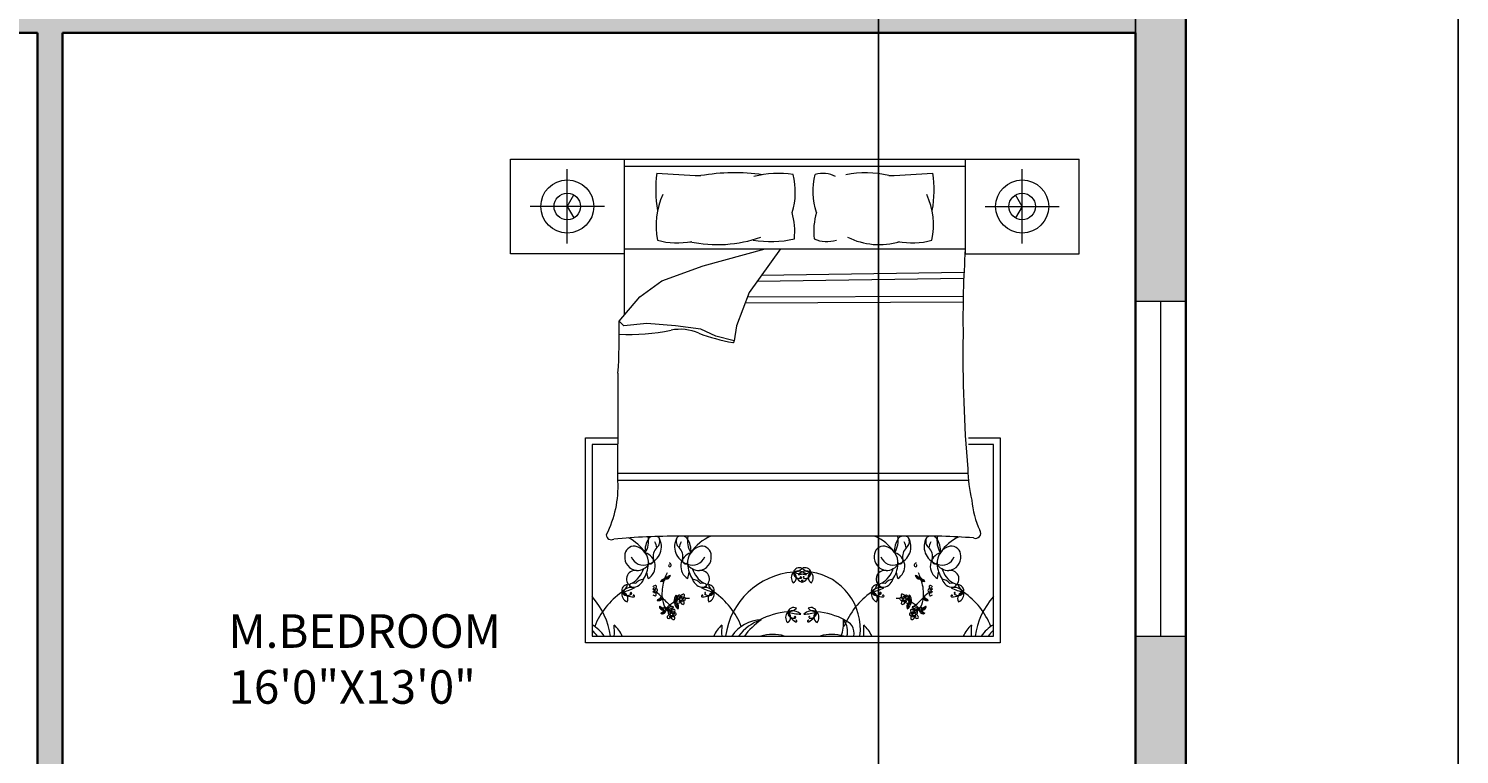
# Model space of a CAD drawing. Units: inches. Extents: x -26 to 13070, y -956 to 6917.
# Tile 5 of 13: x 341 to 597, y -596 to -466. Entities that reach past the tile are written whole.
import ezdxf

# ---------------------------------------------------------------- set-up
doc = ezdxf.new("R2010")
doc.units = ezdxf.units.IN
doc.header["$MEASUREMENT"] = 0
for name, color, linetype, lineweight in [('A-ANNO-DIMS', 2, 'Continuous', 18), ('A-AREA-IDEN', 7, 'Continuous', 18), ('A-FURN', 8, 'Continuous', 13), ('A-GLAZ', 4, 'Continuous', 18), ('A-WALL', 7, 'Continuous', 35), ('A-WALL-PATT', 252, 'Continuous', 13)]:
    doc.layers.add(name, color=color, linetype=linetype, lineweight=lineweight)
doc.styles.get("Standard").update_dxf_attribs({"font": 'arial.ttf'})
doc.dimstyles.get("Standard").update_dxf_attribs({"dimtxt": 0.18, "dimasz": 0.18, "dimexe": 0.18, "dimexo": 0.0625, "dimgap": 0.09, "dimtad": 0, "dimtih": 1, "dimtoh": 1, "dimdec": 0, "dimzin": 0, "dimdsep": 46, "dimlunit": 3, "dimtxsty": 'Standard', "dimcen": 0.09, "dimadec": 0, "dimazin": 0, "dimtfac": 1, "dimtdec": 0, "dimtofl": 0, "dimtmove": 0, "dimatfit": 3, "dimfxl": 1, "dimtolj": 1, "dimtzin": 0, "dimarcsym": 0})

# ---------------------------------------------------------------- blocks, each defined once
blk = doc.blocks.new('WIN-60')
for p, q in [((0, 0), (0, 60)), ((0, 60), (9, 60)), ((4.5, 0), (4.5, 60)), ((9, 60), (9, 0)), ((9, 0), (0, 0))]:
    blk.add_line(p, q)
blk = doc.blocks.new('*D46')
at = {"layer": 'A-ANNO-DIMS', "color": 0, "lineweight": -2, "transparency": 16777216}
for p, q in [((538.7, -457.54), (596.57, -457.54)), ((596.39, -457.72), (596.39, -665.86)), ((596.39, -874.36), (596.39, -666.22)), ((547.7, -874.54), (596.57, -874.54))]:
    blk.add_line(p, q, dxfattribs=at)
at = {"layer": 'A-ANNO-DIMS', "color": 0, "transparency": 16777216}
for points in [[(596.36, -457.72), (596.42, -457.72), (596.39, -457.54)], [(596.36, -874.36), (596.42, -874.36), (596.39, -874.54)]]:
    blk.add_solid(points, dxfattribs=at)
at = {"layer": 'Defpoints', "color": 0, "transparency": 16777216}
for p in [(538.64, -457.54), (596.39, -457.54), (547.64, -874.54)]:
    blk.add_point(p, dxfattribs=at)
at = {"layer": 'A-ANNO-DIMS', "color": 0, "transparency": 16777216, "insert": (596.39, -666.04), "char_height": 0.18, "attachment_point": 5}
blk.add_mtext('\\A1;417', dxfattribs=at)
blk = doc.blocks.new('*D53')
at = {"layer": 'A-ANNO-DIMS', "color": 0, "lineweight": -2, "transparency": 16777216}
for p, q in [((492.64, -622.48), (492.64, 116.39)), ((492.82, 116.21), (515.42, 116.21)), ((538.46, 116.21), (515.86, 116.21)), ((538.64, -622.48), (538.64, 116.39))]:
    blk.add_line(p, q, dxfattribs=at)
at = {"layer": 'A-ANNO-DIMS', "color": 0, "transparency": 16777216}
for points in [[(492.82, 116.24), (492.82, 116.18), (492.64, 116.21)], [(538.46, 116.24), (538.46, 116.18), (538.64, 116.21)]]:
    blk.add_solid(points, dxfattribs=at)
at = {"layer": 'Defpoints', "color": 0, "transparency": 16777216}
for p in [(538.64, 116.21), (492.64, -622.54), (538.64, -622.54)]:
    blk.add_point(p, dxfattribs=at)
at = {"layer": 'A-ANNO-DIMS', "color": 0, "transparency": 16777216, "insert": (515.64, 116.21), "char_height": 0.18, "attachment_point": 5}
blk.add_mtext('\\A1;46', dxfattribs=at)

msp = doc.modelspace()

# ---------------------------------------------------------------- hatches: boundary and pattern name
at = {"layer": 'A-WALL-PATT'}
h = msp.add_hatch(color=256, dxfattribs=at)
h.dxf.hatch_style = 1
h.paths.add_polyline_path([(223.641, 10.458), (214.641, 10.458), (22.641, 10.458), (22.641, -171.042), (31.641, -171.042), (31.641, -135.042), (205.641, -135.042), (205.641, -241.042), (210.141, -241.042), (210.141, -130.542), (94.641, -130.542), (94.641, -76.542), (85.641, -76.542), (85.641, -126.042), (27.141, -126.042), (27.141, 5.958), (85.641, 5.958), (85.641, -52.542), (94.641, -52.542), (94.641, 1.458), (214.641, 1.458), (214.641, -16.542), (223.641, -16.542), (229.641, -16.542), (229.641, -7.542), (223.641, -7.542)])
h.paths.add_polyline_path([(367.048, 10.458), (346.641, 10.458), (337.641, 10.458), (337.641, -7.542), (331.641, -7.542), (331.641, -16.542), (337.641, -16.542), (342.141, -16.542), (342.141, -128.542), (346.641, -128.542), (346.641, 1.458), (367.048, 1.458)])
h.paths.add_polyline_path([(547.641, 10.458), (403.048, 10.458), (403.048, 1.458), (538.641, 1.458), (538.641, -46.542), (547.641, -46.542)])
h.paths.add_polyline_path([(547.641, -106.542), (538.641, -106.542), (538.641, -154.542), (481.013, -154.542), (481.013, -159.042), (538.641, -159.042), (547.641, -159.042)])
h.paths.add_polyline_path([(457.013, -154.542), (342.141, -154.542), (342.141, -165.042), (346.641, -165.042), (346.641, -159.042), (414.141, -159.042), (414.141, -225.042), (346.641, -225.042), (346.641, -189.042), (342.141, -189.042), (342.141, -234.042), (390.641, -234.042), (390.641, -286.042), (395.141, -286.042), (395.141, -234.042), (456.141, -234.042), (456.141, -312.042), (372.641, -312.042), (372.641, -316.542), (462.641, -316.542), (462.641, -312.042), (460.641, -312.042), (460.641, -234.042), (538.641, -234.042), (547.641, -234.042), (547.641, -195.042), (538.641, -195.042), (538.641, -225.042), (418.641, -225.042), (418.641, -159.042), (457.013, -159.042)])
h.paths.add_polyline_path([(547.641, -270.042), (538.641, -270.042), (538.641, -312.042), (486.641, -312.042), (486.641, -316.542), (538.641, -316.542), (547.641, -316.542)], flags=0)
h.paths.add_polyline_path([(547.641, -456.306), (538.641, -456.306), (538.641, -457.542), (346.641, -457.542), (346.641, -316.542), (346.641, -312.042), (342.141, -312.042), (342.141, -457.542), (145.641, -457.542), (145.641, -466.542), (342.141, -466.542), (342.141, -627.042), (346.641, -627.042), (346.641, -466.542), (538.641, -466.542), (538.641, -514.542), (547.641, -514.542)])
h.paths.add_polyline_path([(466.641, -622.542), (372.641, -622.542), (372.641, -627.042), (388.641, -627.042), (388.641, -721.542), (393.141, -721.542), (393.141, -627.042), (462.141, -627.042), (462.141, -717.042), (466.641, -717.042)])
h.paths.add_polyline_path([(547.641, -574.542), (538.641, -574.542), (538.641, -622.542), (492.641, -622.542), (492.641, -627.042), (538.641, -627.042), (538.641, -654.042), (547.641, -654.042)])
h.paths.add_polyline_path([(547.641, -690.042), (538.641, -690.042), (538.641, -717.042), (466.641, -717.042), (466.641, -721.542), (538.641, -721.542), (538.641, -763.542), (547.641, -763.542)])
h.paths.add_polyline_path([(462.141, -717.042), (419.141, -717.042), (419.141, -721.542), (462.141, -721.542)], flags=0)
h.paths.add_polyline_path([(346.641, -721.542), (352.641, -721.542), (352.641, -717.042), (342.141, -717.042), (342.141, -874.542), (342.141, -907.542), (351.141, -907.542), (351.141, -874.542), (395.949, -874.542), (395.949, -865.542), (351.141, -865.542), (351.141, -841.542), (346.641, -841.542)])
h.paths.add_polyline_path([(547.641, -823.542), (538.641, -823.542), (538.641, -865.542), (431.949, -865.542), (431.949, -874.542), (547.641, -874.542)])
h.paths.add_polyline_path([(172.641, -865.713), (140.641, -865.744), (140.641, -788.744), (182.646, -788.704), (182.641, -784.204), (136.141, -784.249), (136.141, -848.332), (131.641, -848.332), (131.641, -874.542), (172.641, -874.542)])
h.paths.add_polyline_path([(217.641, -816.13), (213.141, -816.13), (213.141, -784.174), (208.641, -784.179), (208.641, -865.679), (208.641, -874.542), (217.641, -874.542)])
h.paths.add_polyline_path([(95.641, -865.788), (31.641, -865.849), (31.641, -832.695), (22.641, -832.695), (22.641, -874.542), (95.641, -874.542)])
h.paths.add_polyline_path([(217.641, -741.17), (31.641, -741.349), (31.641, -708.349), (22.641, -708.349), (22.641, -772.542), (22.641, -796.695), (31.641, -796.695), (31.641, -763.542), (31.641, -745.849), (217.641, -745.67)])
h.paths.add_polyline_path([(31.641, -651.349), (99.65, -651.284), (99.641, -642.284), (31.641, -642.349), (31.641, -639.042), (31.641, -588.349), (125.641, -588.259), (125.641, -651.259), (134.641, -651.25), (134.641, -579.25), (112.641, -579.271), (112.641, -549.042), (112.641, -504.271), (85.633, -504.297), (85.641, -513.297), (103.641, -513.28), (103.641, -549.042), (103.641, -579.28), (31.641, -579.349), (31.641, -549.042), (31.641, -513.349), (49.641, -513.314), (49.633, -504.332), (31.641, -504.349), (22.641, -504.358), (22.641, -684.349), (31.641, -684.349)])
h.paths.add_polyline_path([(31.641, -276.042), (145.641, -276.042), (145.641, -402.042), (145.641, -419.542), (154.641, -419.542), (154.641, -411.042), (154.641, -271.542), (210.141, -271.542), (210.141, -265.042), (205.641, -265.042), (205.641, -267.042), (31.641, -267.042), (31.641, -231.042), (22.641, -231.042), (22.641, -426.852), (31.641, -426.852), (31.641, -411.042), (31.641, -402.042)])

# ---------------------------------------------------------------- linework, layer by layer
at = {"layer": 'A-FURN'}
for p, q in [((426.784, -489.112), (528.531, -489.112)), ((436.959, -504.238), (436.959, -490.943)), ((447.133, -489.112), (447.133, -517.038)), ((508.182, -490.418), (447.133, -490.418)), ((518.356, -504.238), (518.356, -490.943)), ((443.606, -497.591), (430.311, -497.591)), ((511.709, -497.591), (525.004, -497.591)), ((447.133, -505.191), (508.182, -505.191)), ((461.266, -508.215), (472.361, -505.191)), ((475.085, -505.191), (469.51, -512.952)), ((453.847, -510.892), (461.266, -508.215)), ((507.909, -509.418), (471.684, -509.926)), ((449.932, -513.776), (453.847, -510.892)), ((507.869, -510.462), (470.924, -510.984)), ((446.222, -518.101), (449.932, -513.776)), ((469.51, -512.952), (467.243, -518.924)), ((507.816, -513.666), (469.18, -513.819)), ((507.822, -514.71), (468.781, -514.87)), ((447.047, -518.924), (446.222, -518.101)), ((451.168, -518.513), (447.047, -518.924)), ((456.32, -518.924), (451.168, -518.513)), ((460.854, -519.542), (456.32, -518.924)), ((463.533, -520.778), (460.854, -519.542)), ((467.243, -518.924), (466.831, -521.602)), ((466.831, -521.602), (463.533, -520.778)), ((440.213, -538.989), (445.969, -538.989)), ((440.213, -575.641), (440.213, -538.989)), ((445.967, -540.168), (441.392, -540.168)), ((441.392, -540.168), (441.392, -574.462)), ((513.212, -540.168), (508.727, -540.168)), ((508.749, -538.989), (514.391, -538.989)), ((513.212, -574.462), (513.212, -540.168)), ((514.391, -538.989), (514.391, -575.641)), ((508.644, -545.334), (445.961, -545.334)), ((508.741, -546.604), (445.961, -546.604)), ((498.313, -556.598), (457.002, -556.598)), ((451.419, -564.146), (451.194, -562.997)), ((458.53, -564.146), (458.755, -562.997)), ((496.075, -564.146), (495.85, -562.997)), ((503.186, -564.146), (503.411, -562.997)), ((514.391, -575.641), (440.213, -575.641)), ((441.392, -574.462), (513.212, -574.462))]:
    msp.add_line(p, q, dxfattribs=at)
for points in [[(447.133, -506.07), (426.784, -506.07), (426.784, -489.112)], [(508.182, -489.112), (508.182, -506.07), (528.531, -506.07), (528.531, -489.112)], [(436.959, -497.591), (438.146, -495.535)], [(518.356, -497.591), (517.169, -495.535)], [(436.959, -497.591), (438.146, -499.647)], [(518.356, -497.591), (517.169, -499.647)]]:
    msp.add_lwpolyline(points, dxfattribs=at)
for points in [[(452.977, -491.648, 0.0748968), (453.101, -498.294, -0.4728166)], [(477.181, -498.665, 0.1409896), (477.384, -491.885, 0.2352448)], [(481.526, -498.665, -0.1409896), (481.322, -491.885, -0.2352448)], [(502.338, -491.648, -0.0748968), (502.214, -498.294, 0.4728166)], [(446.009, -527.417, 0.0012423), (445.961, -546.723, -0.1272016), (443.921, -556.344)], [(508.616, -544.533, 0.0561118), (509.354, -550.131, 0.0953413), (510.784, -555.524)]]:
    msp.add_lwpolyline(points, format="xyb", dxfattribs=at)
for centre, radius in [((436.959, -497.591), 4.748), ((518.356, -497.591), 4.748), ((436.959, -497.591), 2.374), ((518.356, -497.591), 2.374), ((457.297, -567.833), 0.259), ((497.308, -567.833), 0.259), ((455.602, -570.565), 0.259), ((499.002, -570.565), 0.259)]:
    msp.add_circle(centre, radius, dxfattribs=at)
for centre, radius, start, end in [((466.919, -528.466), 36.901, 82.21958, 99.49698), ((490.261, -509.451), 17.886, 76.34271, 101.1841), ((509.06, 476.65), 969.921, 266.685209, 267.149775), ((474.712, -509.817), 18.13, 81.52493, 103.95996), ((482.718, -496.721), 5.033, 63.34374, 106.10256), ((446.255, 476.65), 969.921, 272.850225, 273.314791), ((465.94, -500.962), 13.114, 155.1316, 191.75834), ((489.375, -500.962), 13.114, 348.24166, 24.8684), ((465.187, -502.066), 12.467, 354.01289, 15.82928), ((493.52, -502.066), 12.467, 164.17072, 185.98711), ((456.607, -490.457), 13.635, 255.10393, 281.03689), ((463.785, -480.765), 23.649, 258.03974, 289.26152), ((473.359, -485.928), 17.943, 259.86169, 283.62376), ((483.399, -498.477), 5.394, 245.01826, 288.54073), ((492.823, -491.462), 12.952, 243.87611, 286.17464), ((498.708, -490.457), 13.635, 258.96311, 284.89607), ((690.581, -517.626), 182.823, 176.09997, 180.92818), ((352.931, -520.63), 93.326, 355.82941, 1.55305), ((447.964, -482.07), 38.401, 267.45188, 281.3392), ((457.142, -527.842), 8.282, 66.26158, 101.3392), ((473.895, -483.153), 39.459, 250.11942, 259.33829), ((466.599, -521.685), 0.246, 268.86235, 19.75363), ((746.238, -524.273), 238.484, 179.11454, 184.87351), ((510.014, -556.04), 0.927, 246.52186, 33.82642), ((444.858, -556.279), 0.939, 183.97998, 297.34124), ((455.788, -662.511), 105.92, 89.34325, 95.68869), ((444.461, -563.763), 7.701, 33.66712, 63.29966), ((454.781, -559.181), 3.924, 145.78505, 184.73037), ((447.285, -557.351), 4.215, 328.82178, 9.15542), ((452.506, -557.724), 1.225, 120.0293, 142.32497), ((450.55, -558.446), 3.242, 289.28218, 29.1751), ((450.061, -559.033), 2.925, 7.43599, 29.91487), ((451.989, -557.481), 1.522, 311.56531, 23.83541), ((452.506, -557.724), 1.225, 44.45169, 63.55801), ((459.399, -558.446), 3.242, 150.8249, 250.71782), ((457.961, -557.481), 1.522, 156.16459, 228.43469), ((457.443, -557.724), 1.225, 113.22901, 135.54831), ((459.889, -559.033), 2.925, 150.08513, 172.56401), ((457.443, -557.724), 1.225, 37.67503, 66.71436), ((455.168, -559.181), 3.924, 355.26963, 34.21495), ((462.664, -557.351), 4.215, 169.71335, 211.17822), ((465.488, -563.763), 7.701, 111.49413, 146.33288), ((489.116, -563.763), 7.701, 33.66712, 68.50587), ((499.437, -559.181), 3.924, 145.78505, 184.73037), ((491.941, -557.351), 4.215, 328.82178, 10.28665), ((497.162, -557.724), 1.225, 113.28564, 142.32497), ((495.206, -558.446), 3.242, 289.28218, 29.1751), ((494.716, -559.033), 2.925, 7.43599, 29.91487), ((497.162, -557.724), 1.225, 44.45169, 66.71436), ((496.644, -557.481), 1.522, 311.56531, 23.83541), ((501.429, -655.557), 99.008, 85.24024, 91.80351), ((504.055, -558.446), 3.242, 150.8249, 250.71782), ((502.616, -557.481), 1.522, 156.16459, 228.43469), ((502.098, -557.724), 1.225, 106.63434, 135.54831), ((504.544, -559.033), 2.925, 150.08513, 172.56401), ((502.098, -557.724), 1.225, 37.67503, 72.58143), ((499.823, -559.181), 3.924, 355.26963, 34.21495), ((507.32, -557.351), 4.215, 169.24899, 211.17822), ((510.144, -563.763), 7.701, 113.64533, 146.33288), ((449.651, -560.311), 2.431, 174.94485, 262.88575), ((448.947, -560.066), 1.718, 84.48557, 181.05378), ((450.607, -559.39), 2.361, 201.58187, 291.42215), ((448.419, -561.337), 3.06, 355.29334, 76.921), ((450.158, -561.954), 2.53, 299.90854, 73.1337), ((451.76, -560.891), 0.632, 257.30406, 15.14713), ((454.383, -560.181), 2.086, 131.56531, 195.14713), ((455.567, -560.181), 2.086, 344.85287, 48.43469), ((459.791, -561.954), 2.53, 106.8663, 240.09146), ((458.19, -560.891), 0.632, 164.85287, 282.69594), ((461.53, -561.337), 3.06, 103.079, 184.70666), ((459.342, -559.39), 2.361, 248.57785, 338.41813), ((460.298, -560.311), 2.431, 277.11425, 5.05515), ((461.002, -560.066), 1.718, 358.94622, 95.51443), ((494.307, -560.311), 2.431, 174.94485, 262.88575), ((493.602, -560.066), 1.718, 84.48557, 181.05378), ((495.263, -559.39), 2.361, 201.58187, 291.42215), ((493.075, -561.337), 3.06, 355.29334, 76.921), ((494.814, -561.954), 2.53, 299.90854, 73.1337), ((496.415, -560.891), 0.632, 257.30406, 15.14713), ((499.038, -560.181), 2.086, 131.56531, 195.14713), ((500.222, -560.181), 2.086, 344.85287, 48.43469), ((504.447, -561.954), 2.53, 106.8663, 240.09146), ((502.845, -560.891), 0.632, 164.85287, 282.69594), ((506.186, -561.337), 3.06, 103.079, 184.70666), ((503.998, -559.39), 2.361, 248.57785, 338.41813), ((504.954, -560.311), 2.431, 277.11425, 5.05515), ((505.658, -560.066), 1.718, 358.94622, 95.51443), ((449.092, -564.229), 1.527, 80.26398, 250.86884), ((446.064, -560.868), 4.804, 301.26137, 341.7045), ((449.228, -559.771), 2.956, 272.3591, 324.04014), ((446.019, -561.255), 5.46, 326.28828, 356.5076), ((454.781, -559.181), 3.924, 212.70113, 216.34448), ((462.319, -566.97), 8.427, 153.0032, 159.89408), ((455.267, -561.849), 0.196, 102.70507, 280.43845), ((455.244, -561.728), 0.319, 280.43845, 100.41356), ((455.168, -559.181), 3.924, 323.65552, 327.29887), ((460.721, -559.771), 2.956, 215.95986, 267.6409), ((463.93, -561.255), 5.46, 183.4924, 213.71172), ((463.885, -560.868), 4.804, 198.2955, 238.73863), ((460.857, -564.229), 1.527, 289.13116, 99.73602), ((478.448, -576.253), 13.287, 94.46233, 172.25504), ((478.506, -563.996), 1.473, 137.78732, 219.11446), ((476.833, -563.951), 1.11, 298.5391, 58.36268), ((478.501, -563.049), 1.087, 177.75849, 283.85198), ((478.472, -563.313), 1.101, 63.02737, 163.80375), ((477.357, -560.737), 2.269, 271.45846, 315.37266), ((478.279, -564.92), 2.101, 45.54113, 114.31008), ((480.195, -554.137), 9.295, 252.59304, 267.25817), ((480.593, -561.917), 3.36, 198.91595, 238.01098), ((479.717, -564.92), 2.101, 65.68992, 134.45887), ((477.801, -554.137), 9.295, 272.74183, 287.40696), ((479.524, -563.313), 1.101, 16.19625, 116.97263), ((480.64, -560.737), 2.269, 224.62734, 268.54154), ((477.403, -561.917), 3.36, 301.98902, 341.08405), ((479.496, -563.049), 1.087, 256.14802, 2.24151), ((481.164, -563.951), 1.11, 121.63732, 241.4609), ((479.49, -563.996), 1.473, 320.88554, 42.21268), ((479.119, -573.184), 10.283, 352.86355, 81.81966), ((493.748, -564.229), 1.527, 80.26398, 250.86884), ((490.72, -560.868), 4.804, 301.26137, 341.7045), ((493.884, -559.771), 2.956, 272.3591, 324.04014), ((490.675, -561.255), 5.46, 326.28828, 356.5076), ((499.437, -559.181), 3.924, 212.70113, 216.34448), ((499.361, -561.728), 0.319, 79.58644, 259.56155), ((499.338, -561.849), 0.196, 259.56155, 77.29493), ((492.286, -566.97), 8.427, 20.10592, 26.9968), ((499.823, -559.181), 3.924, 323.65552, 327.29887), ((505.376, -559.771), 2.956, 215.95986, 267.6409), ((508.586, -561.255), 5.46, 183.4924, 213.71172), ((508.541, -560.868), 4.804, 198.2955, 238.73863), ((505.513, -564.229), 1.527, 289.13116, 99.73602), ((447.798, -566.34), 1.101, 92.95159, 193.72796), ((445.547, -564.664), 2.269, 301.38267, 345.29688), ((448.433, -567.829), 2.101, 75.46535, 144.23429), ((444.714, -557.527), 9.295, 282.51726, 297.18239), ((448.778, -565.884), 0.936, 63.97555, 143.26805), ((448.725, -563.77), 1.907, 265.96902, 344.3045), ((450.779, -566.305), 2.031, 96.1662, 141.58255), ((452.632, -565.892), 0.432, 101.56373, 142.6358), ((452.576, -566.048), 0.247, 91.10805, 181.86747), ((452.285, -565.554), 0.623, 288.72627, 352.50315), ((452.71, -565.584), 0.2, 345.23556, 144.9248), ((454.143, -564.88), 0.534, 101.32561, 154.46214), ((453.375, -563.067), 1.608, 280.25878, 300.65599), ((453.745, -561.781), 2.869, 268.32639, 277.13024), ((462.319, -566.97), 8.427, 163.58418, 183.82768), ((453.027, -563.071), 1.635, 308.21012, 316.30712), ((454.03, -564.145), 0.488, 278.34322, 4.28685), ((453.76, -563.717), 0.853, 300.65599, 332.63414), ((454.4, -564.28), 0.207, 55.76575, 157.44165), ((454.723, -564.087), 0.207, 84.37838, 186.05427), ((454.529, -563.256), 0.853, 269.18588, 301.16403), ((454.779, -563.697), 0.488, 237.53317, 323.47681), ((454.306, -562.305), 1.635, 285.51291, 293.60991), ((455.373, -564.143), 0.534, 87.35788, 140.49441), ((454.138, -562.61), 1.608, 301.16403, 321.56124), ((452.83, -562.329), 2.869, 324.68979, 333.49364), ((459.17, -566.305), 2.031, 38.41745, 83.8338), ((461.224, -563.77), 1.907, 195.6955, 274.03098), ((461.172, -565.884), 0.936, 36.73195, 116.02445), ((461.516, -567.829), 2.101, 35.76571, 104.53465), ((465.235, -557.527), 9.295, 242.81761, 257.48274), ((462.151, -566.34), 1.101, 346.27204, 87.04841), ((464.403, -564.664), 2.269, 194.70312, 238.61733), ((478.727, -563.964), 0.144, 283.85198, 219.92454), ((478.901, -564.627), 0.165, 238.01098, 71.55918), ((478.928, -564.546), 0.0802, 71.55918, 188.01668), ((479.096, -564.627), 0.165, 108.44082, 301.98902), ((479.069, -564.546), 0.0802, 351.98332, 108.44082), ((479.256, -563.909), 0.0866, 320.19092, 256.02088), ((492.454, -566.34), 1.101, 92.95159, 193.72796), ((490.202, -564.664), 2.269, 301.38267, 345.29688), ((493.088, -567.829), 2.101, 75.46535, 144.23429), ((489.369, -557.527), 9.295, 282.51726, 297.18239), ((493.433, -565.884), 0.936, 63.97555, 143.26805), ((493.381, -563.77), 1.907, 265.96902, 344.3045), ((495.435, -566.305), 2.031, 96.1662, 141.58255), ((499.232, -564.143), 0.534, 39.50559, 92.64212), ((500.467, -562.61), 1.608, 218.43876, 238.83597), ((501.775, -562.329), 2.869, 206.50636, 215.31021), ((499.826, -563.697), 0.488, 216.52319, 302.46683), ((500.076, -563.256), 0.853, 238.83597, 270.81412), ((500.299, -562.305), 1.635, 246.39009, 254.48709), ((499.882, -564.087), 0.207, 353.94573, 95.62162), ((500.575, -564.145), 0.488, 175.71315, 261.65678), ((500.204, -564.28), 0.207, 22.55835, 124.23425), ((500.845, -563.717), 0.853, 207.36586, 239.34401), ((492.286, -566.97), 8.427, 356.17232, 16.41582), ((501.578, -563.071), 1.635, 223.69288, 231.78988), ((501.23, -563.067), 1.608, 239.34401, 259.74122), ((500.86, -561.781), 2.869, 262.86976, 271.67361), ((500.462, -564.88), 0.534, 25.53786, 78.67439), ((501.895, -565.584), 0.2, 35.0752, 194.76444), ((502.319, -565.554), 0.623, 187.49685, 251.27373), ((502.029, -566.048), 0.247, 358.13253, 88.89195), ((501.972, -565.892), 0.432, 37.3642, 78.43627), ((505.879, -563.77), 1.907, 195.6955, 274.03098), ((503.825, -566.305), 2.031, 38.41745, 83.8338), ((505.827, -565.884), 0.936, 36.73195, 116.02445), ((506.172, -567.829), 2.101, 35.76571, 104.53465), ((509.891, -557.527), 9.295, 242.81761, 257.48274), ((509.058, -564.664), 2.269, 194.70312, 238.61733), ((506.807, -566.34), 1.101, 346.27204, 87.04841), ((431.501, -576.253), 13.287, 7.74496, 41.8856), ((454.232, -577.566), 13.287, 124.38655, 158.59079), ((448.168, -566.915), 1.473, 167.71153, 249.03868), ((446.695, -567.71), 1.11, 328.46331, 88.28689), ((448.94, -564.071), 3.36, 228.84017, 267.9352), ((447.691, -566.096), 1.087, 207.6827, 313.77619), ((448.343, -566.777), 0.144, 313.77619, 249.71835), ((448.808, -567.181), 0.0802, 101.4834, 217.94089), ((448.825, -567.265), 0.165, 267.9352, 101.4834), ((452.274, -566.293), 0.259, 273.27684, 86.72316), ((452.627, -566.773), 0.428, 217.76209, 259.04026), ((453.089, -566.203), 0.787, 203.42757, 227.61037), ((452.839, -566.546), 0.536, 80.3487, 133.65382), ((452.743, -566.103), 0.424, 229.78892, 317.67915), ((452.265, -567.001), 0.602, 355.05304, 68.36176), ((452.737, -567.103), 0.848, 83.08516, 105.71709), ((452.667, -567.036), 0.199, 232.47371, 355.05304), ((446.863, -574.14), 9.661, 43.15413, 52.0459), ((452.891, -566.238), 0.223, 317.67915, 80.3487), ((453.537, -568.303), 0.534, 101.32561, 154.46214), ((452.768, -566.491), 1.608, 280.25878, 300.65599), ((453.139, -565.205), 2.869, 268.32639, 277.13024), ((452.421, -566.495), 1.635, 308.21012, 316.30712), ((453.424, -567.569), 0.488, 278.34322, 4.28685), ((453.154, -567.14), 0.853, 300.65599, 332.63414), ((453.794, -567.704), 0.207, 55.76575, 157.44165), ((458.121, -567.182), 4.225, 184.75602, 209.20408), ((464.203, -558.187), 13.902, 222.24124, 232.17444), ((455.944, -567.712), 0.718, 272.84988, 356.12261), ((455.314, -567.448), 1.181, 304.53686, 16.36991), ((455.437, -567.991), 0.695, 321.76073, 7.92519), ((456.953, -567.78), 0.836, 127.31045, 187.92519), ((456.149, -569.112), 0.718, 20.5253, 88.5375), ((455.806, -567.686), 0.858, 355.01064, 41.65801), ((456.753, -568.32), 0.257, 148.0499, 225.62681), ((458.556, -572.793), 5.068, 113.05007, 113.84774), ((457.228, -568.616), 0.817, 104.75581, 148.0499), ((456.77, -568.031), 0.511, 247.40857, 351.43859), ((457.011, -567.473), 0.353, 126.10456, 271.42811), ((456.972, -567.377), 0.254, 353.75256, 131.70535), ((456.914, -568.052), 0.172, 262.90601, 7.13198), ((456.733, -567.679), 0.357, 0.06451, 61.15075), ((456.818, -567.375), 0.408, 311.84125, 355.78771), ((457.65, -568.313), 0.428, 151.21959, 259.04026), ((457.656, -567.432), 0.432, 101.56373, 176.36503), ((457.599, -567.588), 0.247, 91.10805, 181.86747), ((458.112, -567.743), 0.787, 203.42757, 227.61037), ((457.862, -568.086), 0.536, 80.3487, 133.65382), ((457.766, -567.643), 0.424, 229.78892, 317.67915), ((457.309, -567.093), 0.623, 288.72627, 352.50315), ((457.288, -568.541), 0.602, 355.05304, 68.36176), ((457.761, -568.643), 0.848, 83.08516, 105.71709), ((457.733, -567.124), 0.2, 345.23556, 144.9248), ((457.915, -567.778), 0.223, 317.67915, 80.3487), ((458.556, -572.793), 5.068, 87.10709, 94.75853), ((461.124, -567.265), 0.165, 78.5166, 272.0648), ((461.009, -564.071), 3.36, 272.0648, 311.15983), ((461.141, -567.181), 0.0802, 322.05911, 78.5166), ((462.258, -566.096), 1.087, 226.22381, 332.3173), ((461.622, -566.723), 0.0866, 290.26671, 226.22708), ((463.254, -567.71), 1.11, 91.71311, 211.53669), ((461.781, -566.915), 1.473, 290.96132, 12.28847), ((455.717, -577.566), 13.287, 21.40921, 55.61345), ((498.888, -577.566), 13.287, 124.38655, 158.59079), ((492.824, -566.915), 1.473, 167.71153, 249.03868), ((492.346, -566.096), 1.087, 207.6827, 313.77619), ((493.596, -564.071), 3.36, 228.84017, 267.9352), ((491.351, -567.71), 1.11, 328.46331, 88.28689), ((492.999, -566.777), 0.144, 313.77619, 249.71835), ((493.464, -567.181), 0.0802, 101.4834, 217.94089), ((493.48, -567.265), 0.165, 267.9352, 101.4834), ((496.049, -572.793), 5.068, 85.24147, 92.89291), ((496.69, -567.778), 0.223, 99.6513, 222.32085), ((496.839, -567.643), 0.424, 222.32085, 310.21108), ((496.743, -568.086), 0.536, 46.34618, 99.6513), ((496.872, -567.124), 0.2, 35.0752, 194.76444), ((497.296, -567.093), 0.623, 187.49685, 251.27373), ((497.317, -568.541), 0.602, 111.63824, 184.94696), ((496.844, -568.643), 0.848, 74.28291, 96.91484), ((497.006, -567.588), 0.247, 358.13253, 88.89195), ((496.493, -567.743), 0.787, 312.38963, 336.57243), ((496.949, -567.432), 0.432, 3.63497, 78.43627), ((496.955, -568.313), 0.428, 280.95974, 28.78041), ((497.835, -568.031), 0.511, 188.56141, 292.59143), ((497.633, -567.377), 0.254, 48.29465, 186.24744), ((497.787, -567.375), 0.408, 184.21229, 228.15875), ((497.872, -567.679), 0.357, 118.84925, 179.93549), ((497.691, -568.052), 0.172, 172.86802, 277.09399), ((497.594, -567.473), 0.353, 268.57189, 53.89544), ((497.377, -568.616), 0.817, 31.9501, 75.24419), ((498.456, -569.112), 0.718, 91.4625, 159.4747), ((498.799, -567.686), 0.858, 138.34199, 184.98936), ((498.66, -567.712), 0.718, 183.87739, 267.15012), ((497.852, -568.32), 0.257, 314.37319, 31.9501), ((496.049, -572.793), 5.068, 66.15226, 66.94993), ((499.291, -567.448), 1.181, 163.63009, 235.46314), ((497.651, -567.78), 0.836, 352.07481, 52.68955), ((499.167, -567.991), 0.695, 172.07481, 218.23927), ((490.402, -558.187), 13.902, 307.82556, 317.75876), ((496.484, -567.182), 4.225, 330.79592, 355.24398), ((501.181, -567.569), 0.488, 175.71315, 261.65678), ((507.742, -574.14), 9.661, 127.9541, 136.84587), ((500.811, -567.704), 0.207, 22.55835, 124.23425), ((501.451, -567.14), 0.853, 207.36586, 239.34401), ((502.184, -566.495), 1.635, 223.69288, 231.78988), ((501.836, -566.491), 1.608, 239.34401, 259.74122), ((501.466, -565.205), 2.869, 262.86976, 271.67361), ((501.068, -568.303), 0.534, 25.53786, 78.67439), ((501.714, -566.238), 0.223, 99.6513, 222.32085), ((501.862, -566.103), 0.424, 222.32085, 310.21108), ((501.766, -566.546), 0.536, 46.34618, 99.6513), ((502.34, -567.001), 0.602, 111.63824, 184.94696), ((501.938, -567.036), 0.199, 184.94696, 307.52629), ((501.868, -567.103), 0.848, 74.28291, 96.91484), ((501.516, -566.203), 0.787, 312.38963, 336.57243), ((501.978, -566.773), 0.428, 280.95974, 322.23791), ((502.331, -566.293), 0.259, 93.27684, 266.72316), ((505.78, -567.265), 0.165, 78.5166, 272.0648), ((505.665, -564.071), 3.36, 272.0648, 311.15983), ((505.797, -567.181), 0.0802, 322.05911, 78.5166), ((506.914, -566.096), 1.087, 226.22381, 332.3173), ((506.277, -566.723), 0.0866, 290.26671, 226.22708), ((507.91, -567.71), 1.11, 91.71311, 211.53669), ((506.437, -566.915), 1.473, 290.96132, 12.28847), ((500.373, -577.566), 13.287, 21.40921, 55.61345), ((523.104, -576.253), 13.287, 138.1144, 172.25504), ((453.717, -569.24), 0.289, 146.86359, 236.90213), ((457.796, -562.867), 7.57, 235.1882, 238.88441), ((454.213, -568.821), 0.783, 199.47987, 267.68284), ((454.126, -569.117), 0.675, 212.81548, 277.39917), ((453.734, -569.568), 0.783, 266.97007, 338.29129), ((449.605, -563.978), 7.57, 302.6784, 306.37461), ((453.931, -570.187), 0.289, 214.3538, 304.39233), ((454.039, -569.091), 0.3, 238.88441, 314.26458), ((453.974, -569.762), 0.675, 280.30568, 17.1958), ((453.917, -569.832), 0.3, 306.37461, 21.75478), ((454.405, -569.637), 0.226, 19.36054, 201.75478), ((454.406, -569.468), 0.226, 311.87034, 134.26458), ((458.654, -571.527), 4.513, 153.78194, 158.29129), ((455.063, -568.444), 1.181, 247.23048, 319.06353), ((454.673, -568.841), 0.695, 264.45436, 310.61881), ((455.182, -569.117), 0.718, 218.32082, 298.81623), ((458.121, -567.182), 4.225, 214.00334, 222.49171), ((458.556, -572.793), 5.068, 120.54402, 139.81798), ((455.058, -571.051), 0.257, 148.0499, 225.62681), ((455.533, -571.347), 0.817, 104.75581, 148.0499), ((455.075, -570.762), 0.511, 247.40857, 351.43859), ((455.316, -570.204), 0.353, 126.10456, 271.42811), ((455.277, -570.108), 0.254, 353.75256, 131.70535), ((455.669, -570.003), 0.836, 70.00407, 130.61881), ((455.219, -570.783), 0.172, 262.90601, 7.13198), ((455.038, -570.41), 0.357, 0.06451, 61.15075), ((455.123, -570.106), 0.408, 311.84125, 355.78771), ((455.129, -568.987), 0.858, 297.70426, 344.35163), ((455.956, -571.044), 0.428, 151.21959, 259.04026), ((455.961, -570.163), 0.432, 101.56373, 176.36503), ((455.904, -570.319), 0.247, 91.10805, 181.86747), ((456.417, -570.475), 0.787, 203.42757, 227.61037), ((456.167, -570.817), 0.536, 80.3487, 133.65382), ((456.071, -570.374), 0.424, 229.78892, 317.67915), ((455.614, -569.825), 0.623, 288.72627, 352.50315), ((455.593, -571.272), 0.602, 355.05304, 68.36176), ((456.066, -571.374), 0.848, 83.08516, 105.71709), ((456.038, -569.855), 0.2, 345.23556, 144.9248), ((455.584, -568.99), 0.695, 8.72271, 54.88717), ((455.621, -569.545), 1.181, 0.278, 72.11105), ((456.22, -570.509), 0.223, 317.67915, 80.3487), ((457.096, -568.758), 0.836, 188.72271, 249.33746), ((456.024, -569.177), 0.858, 334.9899, 21.63727), ((457.69, -568.576), 0.199, 232.47371, 355.05304), ((477.431, -583.369), 13.287, 94.46233, 117.4146), ((477.489, -571.113), 1.473, 137.78732, 219.11446), ((475.815, -571.067), 1.11, 298.5391, 58.36268), ((477.455, -570.43), 1.101, 63.02737, 163.80375), ((476.34, -567.854), 2.269, 271.45846, 315.37266), ((477.262, -572.037), 2.101, 45.54113, 114.31008), ((479.576, -569.033), 3.36, 198.91595, 238.01098), ((479.178, -561.253), 9.295, 252.59304, 267.25817), ((477.483, -570.165), 1.087, 177.75849, 283.85198), ((477.709, -571.081), 0.144, 283.85198, 219.92454), ((480.734, -572.037), 2.101, 65.68992, 134.45887), ((478.818, -561.253), 9.295, 272.74183, 287.40696), ((480.541, -570.43), 1.101, 16.19625, 116.97263), ((481.657, -567.854), 2.269, 224.62734, 268.54154), ((480.273, -571.025), 0.0866, 320.19092, 256.02088), ((478.42, -569.033), 3.36, 301.98902, 341.08405), ((480.513, -570.165), 1.087, 256.14802, 2.24151), ((482.181, -571.067), 1.11, 121.63732, 241.4609), ((480.508, -571.113), 1.473, 320.88554, 42.21268), ((480.565, -583.369), 13.287, 62.5854, 85.53767), ((496.915, -568.576), 0.199, 184.94696, 307.52629), ((498.581, -569.177), 0.858, 158.36273, 205.0101), ((498.984, -569.545), 1.181, 107.88895, 179.722), ((497.508, -568.758), 0.836, 290.66254, 351.27729), ((498.385, -570.509), 0.223, 99.6513, 222.32085), ((498.534, -570.374), 0.424, 222.32085, 310.21108), ((499.021, -568.99), 0.695, 125.11283, 171.27729), ((498.438, -570.817), 0.536, 46.34618, 99.6513), ((498.567, -569.855), 0.2, 35.0752, 194.76444), ((498.991, -569.825), 0.623, 187.49685, 251.27373), ((499.011, -571.272), 0.602, 111.63824, 184.94696), ((498.539, -571.374), 0.848, 74.28291, 96.91484), ((496.049, -572.793), 5.068, 40.18202, 59.45598), ((498.936, -570.003), 0.836, 49.38119, 109.99593), ((499.542, -568.444), 1.181, 220.93647, 292.76952), ((499.476, -568.987), 0.858, 195.64837, 242.29574), ((498.7, -570.319), 0.247, 358.13253, 88.89195), ((498.188, -570.475), 0.787, 312.38963, 336.57243), ((498.644, -570.163), 0.432, 3.63497, 78.43627), ((498.649, -571.044), 0.428, 280.95974, 28.78041), ((499.53, -570.762), 0.511, 188.56141, 292.59143), ((499.328, -570.108), 0.254, 48.29465, 186.24744), ((499.482, -570.106), 0.408, 184.21229, 228.15875), ((499.423, -569.117), 0.718, 241.18377, 321.67918), ((499.567, -570.41), 0.357, 118.84925, 179.93549), ((499.386, -570.783), 0.172, 172.86802, 277.09399), ((499.288, -570.204), 0.353, 268.57189, 53.89544), ((499.072, -571.347), 0.817, 31.9501, 75.24419), ((499.932, -568.841), 0.695, 229.38119, 275.54564), ((496.484, -567.182), 4.225, 317.50829, 325.99666), ((499.547, -571.051), 0.257, 314.37319, 31.9501), ((500.631, -569.762), 0.675, 162.8042, 259.69432), ((500.199, -569.468), 0.226, 45.73542, 228.12966), ((500.2, -569.637), 0.226, 338.24522, 160.63946), ((495.95, -571.527), 4.513, 21.70871, 26.21806), ((500.871, -569.568), 0.783, 201.70871, 273.02993), ((500.566, -569.091), 0.3, 225.73542, 301.11559), ((500.688, -569.832), 0.3, 158.24522, 233.62539), ((500.479, -569.117), 0.675, 262.60083, 327.18452), ((500.392, -568.821), 0.783, 272.31716, 340.52013), ((505, -563.978), 7.57, 233.62539, 237.3216), ((500.674, -570.187), 0.289, 235.60767, 325.6462), ((496.808, -562.867), 7.57, 301.11559, 304.8118), ((500.888, -569.24), 0.289, 303.09787, 33.13641), ((438.166, -578.032), 6.474, 33.46172, 60.11157), ((435.837, -579.239), 8.068, 36.30357, 46.48142), ((441.792, -576.534), 5.402, 22.55474, 48.95456), ((426.994, -573.631), 18.383, 357.40811, 3.65191), ((455.995, -571.307), 0.199, 232.47371, 355.05304), ((468.157, -576.534), 5.402, 131.04544, 157.44526), ((482.955, -573.631), 18.383, 176.34809, 182.59189), ((471.783, -578.032), 6.474, 91.27197, 146.53828), ((474.112, -579.239), 8.068, 107.85038, 143.69643), ((478.352, -581.507), 12.001, 124.01234, 144.05304), ((477.883, -571.743), 0.165, 238.01098, 71.55918), ((477.91, -571.663), 0.0802, 71.55918, 188.01668), ((480.113, -571.743), 0.165, 108.44082, 301.98902), ((480.086, -571.663), 0.0802, 351.98332, 108.44082), ((480.448, -572.245), 5.949, 338.11703, 6.61954), ((485.905, -573.901), 2.385, 346.38982, 79.07385), ((484.113, -573.573), 3.016, 342.86088, 41.90487), ((471.65, -573.631), 18.383, 357.40811, 3.65191), ((486.448, -576.534), 5.402, 22.55474, 48.95456), ((498.61, -571.307), 0.199, 184.94696, 307.52629), ((512.813, -576.534), 5.402, 131.04544, 157.44526), ((527.611, -573.631), 18.383, 176.34809, 182.59189), ((516.439, -578.032), 6.474, 119.88843, 146.53828), ((518.768, -579.239), 8.068, 133.51858, 143.69643), ((473.715, -581.448), 7.306, 73.54311, 107.0202), ((476.61, -585.213), 10.804, 94.37872, 95.63574), ((482.3, -592.615), 19.306, 109.72171, 109.90284), ((484.281, -581.448), 7.306, 72.9798, 106.45689), ((481.387, -585.213), 10.804, 84.36426, 85.62128), ((475.696, -592.615), 19.306, 70.09716, 70.27829)]:
    msp.add_arc(centre, radius, start, end, dxfattribs=at)
at = {"layer": 'A-WALL'}
for p, q in [((547.641, 10.458), (547.641, -874.542)), ((342.141, -466.542), (145.641, -466.542)), ((342.141, -466.542), (342.141, -627.042)), ((346.641, -466.542), (538.641, -466.542)), ((346.641, -466.542), (346.641, -627.042)), ((538.641, -466.542), (538.641, -622.542))]:
    msp.add_line(p, q, dxfattribs=at)

# ---------------------------------------------------------------- block references
at = {"layer": 'A-GLAZ'}
msp.add_blockref('WIN-60', (538.641, -574.542), dxfattribs=at)

# ---------------------------------------------------------------- texts
at = {"layer": 'A-AREA-IDEN', "insert": (376.325, -570.545), "char_height": 6, "attachment_point": 1}
msp.add_mtext('M.BEDROOM\\P16\'0"X13\'0"', dxfattribs=at)

# ---------------------------------------------------------------- dimensions: what is measured, and where the dimension line sits
at = {"layer": 'A-ANNO-DIMS'}
dim = msp.add_linear_dim(base=(538.641, 116.209), p1=(492.641, -622.542), p2=(538.641, -622.542), dimstyle='Standard', override={"dimdec": 0, "dimlfac": 1, "dimrnd": 0, "dimzin": 0, "dimdsep": 46, "dimlunit": 2}, dxfattribs=at)
dim.commit()
dim.dimension.update_dxf_attribs({"geometry": '*D53', "text_midpoint": (515.641, 116.209)})
dim = msp.add_linear_dim(base=(596.392, -457.542), p1=(547.641, -874.542), p2=(538.641, -457.542), angle=90, dimstyle='Standard', override={"dimdec": 0, "dimlfac": 1, "dimrnd": 0, "dimzin": 0, "dimdsep": 46, "dimlunit": 2}, dxfattribs=at)
dim.commit()
dim.dimension.update_dxf_attribs({"geometry": '*D46', "text_midpoint": (596.392, -666.042)})

doc.saveas('drawing.dxf')
